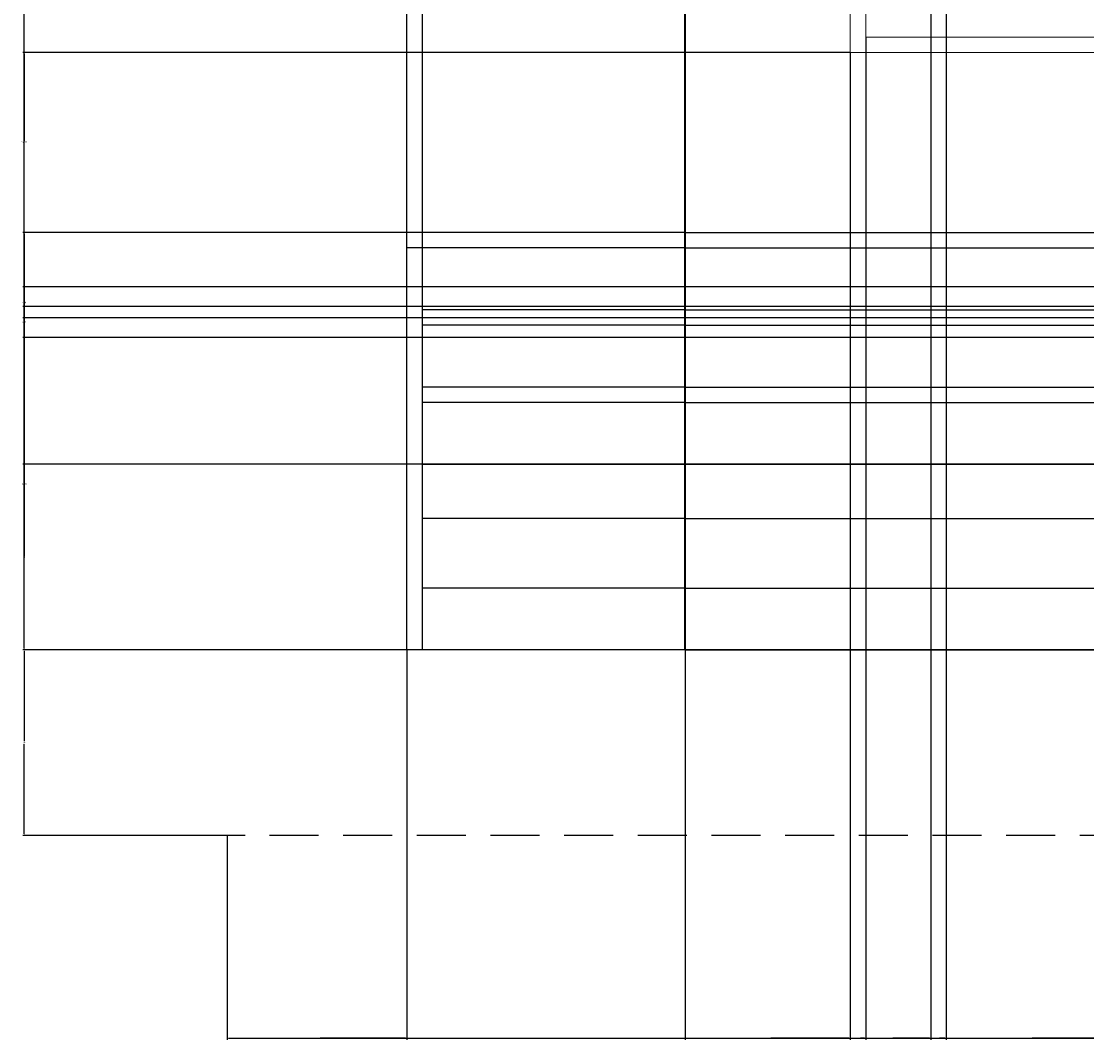
# Model space of a CAD drawing. Units: inches. Extents: x 1817 to 2378, y 1915 to 2370.
# Tile 1 of 8: x 1817 to 1955, y 1915 to 2047. Entities that reach past the tile are written whole.
import ezdxf

# ---------------------------------------------------------------- set-up
doc = ezdxf.new("R2010")
doc.units = ezdxf.units.IN
doc.linetypes.add('DASHED', pattern=[19.05, 12.7, -6.35])
doc.linetypes.add('DASHED2', pattern=[9.525, 6.35, -3.175])
for name, color, linetype, lineweight in [('A-ANNO-DIMS', 2, 'Continuous', 18), ('A-ELEV', 7, 'Continuous', 35), ('A-ELEV-HIDN', 8, 'DASHED', 18), ('A-FLOR-STRS', 3, 'Continuous', 25), ('A-GLAZ', 4, 'Continuous', 18), ('C-TOPO', 8, 'DASHED2', 25)]:
    doc.layers.add(name, color=color, linetype=linetype, lineweight=lineweight)
doc.styles.get("Standard").update_dxf_attribs({"font": 'arial.ttf'})
doc.dimstyles.get("Standard").update_dxf_attribs({"dimtxt": 0.18, "dimasz": 0.18, "dimexe": 0.18, "dimexo": 0.0625, "dimgap": 0.09, "dimtad": 0, "dimtih": 1, "dimtoh": 1, "dimdec": 4, "dimzin": 0, "dimdsep": 46, "dimtxsty": 'Standard', "dimcen": 0.09, "dimadec": 0, "dimazin": 0, "dimtfac": 1, "dimtdec": 4, "dimtofl": 0, "dimtmove": 0, "dimatfit": 3, "dimfxl": 1, "dimtolj": 1, "dimtzin": 0, "dimarcsym": 0})

# ---------------------------------------------------------------- blocks, each defined once
blk = doc.blocks.new('WIN-SQ-900')
for points in [[(1924.43, 2204.58), (1960.43, 2204.58), (1960.43, 2217.58), (1924.43, 2217.58)], [(1924.43, 2204.58), (1960.43, 2204.58), (1960.43, 2168.58), (1924.43, 2168.58)], [(1926.43, 2202.58), (1958.43, 2202.58), (1958.43, 2170.58), (1926.43, 2170.58)]]:
    blk.add_lwpolyline(points, close=True)
blk = doc.blocks.new('*D10')
at = {"layer": 'A-ANNO-DIMS', "color": 0, "lineweight": -2, "transparency": 16777216}
for p, q in [((1867.08, 2019.57), (1867.08, 2369.94)), ((1867.26, 2369.76), (1884.87, 2369.76)), ((1902.9, 2369.76), (1885.3, 2369.76)), ((1903.08, 2019.57), (1903.08, 2369.94))]:
    blk.add_line(p, q, dxfattribs=at)
at = {"layer": 'A-ANNO-DIMS', "color": 0, "transparency": 16777216}
for points in [[(1867.26, 2369.79), (1867.26, 2369.73), (1867.08, 2369.76)], [(1902.9, 2369.79), (1902.9, 2369.73), (1903.08, 2369.76)]]:
    blk.add_solid(points, dxfattribs=at)
at = {"layer": 'Defpoints', "color": 0, "transparency": 16777216}
for p in [(1903.08, 2369.76), (1867.08, 2019.51), (1903.08, 2019.51)]:
    blk.add_point(p, dxfattribs=at)
at = {"layer": 'A-ANNO-DIMS', "color": 0, "transparency": 16777216, "insert": (1885.08, 2369.76), "char_height": 0.18, "attachment_point": 5}
blk.add_mtext('\\A1;36', dxfattribs=at)
blk = doc.blocks.new('*D12')
at = {"layer": 'A-ANNO-DIMS', "color": 0, "lineweight": -2, "transparency": 16777216}
for p, q in [((1924.43, 2042.72), (1924.43, 1915.08)), ((1903.08, 2019.45), (1903.08, 1915.08)), ((1903.26, 1915.26), (1913.36, 1915.26)), ((1924.25, 1915.26), (1914.15, 1915.26))]:
    blk.add_line(p, q, dxfattribs=at)
at = {"layer": 'A-ANNO-DIMS', "color": 0, "transparency": 16777216}
for points in [[(1903.26, 1915.29), (1903.26, 1915.23), (1903.08, 1915.26)], [(1924.25, 1915.29), (1924.25, 1915.23), (1924.43, 1915.26)]]:
    blk.add_solid(points, dxfattribs=at)
at = {"layer": 'Defpoints', "color": 0, "transparency": 16777216}
for p in [(1924.43, 2042.79), (1903.08, 2019.51), (1924.43, 1915.26)]:
    blk.add_point(p, dxfattribs=at)
at = {"layer": 'A-ANNO-DIMS', "color": 0, "transparency": 16777216, "insert": (1913.76, 1915.26), "char_height": 0.18, "attachment_point": 5}
blk.add_mtext('\\A1;21.34', dxfattribs=at)
blk = doc.blocks.new('*D13')
at = {"layer": 'A-ANNO-DIMS', "color": 0, "lineweight": -2, "transparency": 16777216}
for p, q in [((1934.83, 2100.21), (1934.83, 1915.08)), ((1924.43, 2042.72), (1924.43, 1915.08)), ((1924.61, 1915.26), (1929.31, 1915.26)), ((1934.65, 1915.26), (1929.94, 1915.26))]:
    blk.add_line(p, q, dxfattribs=at)
at = {"layer": 'A-ANNO-DIMS', "color": 0, "transparency": 16777216}
for points in [[(1924.61, 1915.29), (1924.61, 1915.23), (1924.43, 1915.26)], [(1934.65, 1915.29), (1934.65, 1915.23), (1934.83, 1915.26)]]:
    blk.add_solid(points, dxfattribs=at)
at = {"layer": 'Defpoints', "color": 0, "transparency": 16777216}
for p in [(1934.83, 2100.28), (1924.43, 2042.79), (1934.83, 1915.26)]:
    blk.add_point(p, dxfattribs=at)
at = {"layer": 'A-ANNO-DIMS', "color": 0, "transparency": 16777216, "insert": (1929.63, 1915.26), "char_height": 0.18, "attachment_point": 5}
blk.add_mtext('\\A1;10.4', dxfattribs=at)
blk = doc.blocks.new('*D14')
at = {"layer": 'A-ANNO-DIMS', "color": 0, "lineweight": -2, "transparency": 16777216}
for p, q in [((1934.83, 2100.21), (1934.83, 1915.08)), ((1960.43, 2042.72), (1960.43, 1915.08)), ((1935.01, 1915.26), (1947.3, 1915.26)), ((1960.25, 1915.26), (1947.95, 1915.26))]:
    blk.add_line(p, q, dxfattribs=at)
at = {"layer": 'A-ANNO-DIMS', "color": 0, "transparency": 16777216}
for points in [[(1935.01, 1915.29), (1935.01, 1915.23), (1934.83, 1915.26)], [(1960.25, 1915.29), (1960.25, 1915.23), (1960.43, 1915.26)]]:
    blk.add_solid(points, dxfattribs=at)
at = {"layer": 'Defpoints', "color": 0, "transparency": 16777216}
for p in [(1934.83, 2100.28), (1960.43, 2042.79), (1960.43, 1915.26)]:
    blk.add_point(p, dxfattribs=at)
at = {"layer": 'A-ANNO-DIMS', "color": 0, "transparency": 16777216, "insert": (1947.63, 1915.26), "char_height": 0.18, "attachment_point": 5}
blk.add_mtext('\\A1;25.6', dxfattribs=at)
blk = doc.blocks.new('*D23')
at = {"layer": 'A-ANNO-DIMS', "color": 0, "lineweight": -2, "transparency": 16777216}
for p, q in [((2320.11, 2156.45), (2320.11, 1915.08)), ((1867.08, 1965.45), (1867.08, 1915.08)), ((1867.26, 1915.26), (2093.3, 1915.26)), ((2319.93, 1915.26), (2093.89, 1915.26))]:
    blk.add_line(p, q, dxfattribs=at)
at = {"layer": 'A-ANNO-DIMS', "color": 0, "transparency": 16777216}
for points in [[(1867.26, 1915.29), (1867.26, 1915.23), (1867.08, 1915.26)], [(2319.93, 1915.29), (2319.93, 1915.23), (2320.11, 1915.26)]]:
    blk.add_solid(points, dxfattribs=at)
at = {"layer": 'Defpoints', "color": 0, "transparency": 16777216}
for p in [(2320.11, 2156.51), (1867.08, 1965.51), (2320.11, 1915.26)]:
    blk.add_point(p, dxfattribs=at)
at = {"layer": 'A-ANNO-DIMS', "color": 0, "transparency": 16777216, "insert": (2093.6, 1915.26), "char_height": 0.18, "attachment_point": 5}
blk.add_mtext('\\A1;453', dxfattribs=at)
blk = doc.blocks.new('*D53')
at = {"layer": 'A-ANNO-DIMS', "color": 0, "lineweight": -2, "transparency": 16777216}
for p, q in [((1867.02, 1965.51), (1817.4, 1965.51)), ((1817.58, 1965.33), (1817.58, 1953.69)), ((1817.58, 1941.69), (1817.58, 1953.33)), ((1843.77, 1941.51), (1817.4, 1941.51))]:
    blk.add_line(p, q, dxfattribs=at)
at = {"layer": 'A-ANNO-DIMS', "color": 0, "transparency": 16777216}
for points in [[(1817.55, 1965.33), (1817.61, 1965.33), (1817.58, 1965.51)], [(1817.55, 1941.69), (1817.61, 1941.69), (1817.58, 1941.51)]]:
    blk.add_solid(points, dxfattribs=at)
at = {"layer": 'Defpoints', "color": 0, "transparency": 16777216}
for p in [(1817.58, 1965.51), (1867.08, 1965.51), (1843.83, 1941.51)]:
    blk.add_point(p, dxfattribs=at)
at = {"layer": 'A-ANNO-DIMS', "color": 0, "transparency": 16777216, "insert": (1817.58, 1953.51), "char_height": 0.18, "attachment_point": 5}
blk.add_mtext('\\A1;24', dxfattribs=at)
blk = doc.blocks.new('*D54')
at = {"layer": 'A-ANNO-DIMS', "color": 0, "lineweight": -2, "transparency": 16777216}
for p, q in [((1901.02, 2343.51), (1817.4, 2343.51)), ((1817.58, 2343.33), (1817.58, 2154.69)), ((1817.58, 1965.69), (1817.58, 2154.33)), ((1867.02, 1965.51), (1817.4, 1965.51))]:
    blk.add_line(p, q, dxfattribs=at)
at = {"layer": 'A-ANNO-DIMS', "color": 0, "transparency": 16777216}
for points in [[(1817.55, 2343.33), (1817.61, 2343.33), (1817.58, 2343.51)], [(1817.55, 1965.69), (1817.61, 1965.69), (1817.58, 1965.51)]]:
    blk.add_solid(points, dxfattribs=at)
at = {"layer": 'Defpoints', "color": 0, "transparency": 16777216}
for p in [(1817.58, 2343.51), (1901.08, 2343.51), (1867.08, 1965.51)]:
    blk.add_point(p, dxfattribs=at)
at = {"layer": 'A-ANNO-DIMS', "color": 0, "transparency": 16777216, "insert": (1817.58, 2154.51), "char_height": 0.18, "attachment_point": 5}
blk.add_mtext('\\A1;378', dxfattribs=at)
blk = doc.blocks.new('*D55')
at = {"layer": 'A-ANNO-DIMS', "color": 0, "lineweight": -2, "transparency": 16777216}
for p, q in [((1903.02, 1989.51), (1817.4, 1989.51)), ((1817.58, 1989.33), (1817.58, 1977.69)), ((1817.58, 1965.69), (1817.58, 1977.33)), ((1867.02, 1965.51), (1817.4, 1965.51))]:
    blk.add_line(p, q, dxfattribs=at)
at = {"layer": 'A-ANNO-DIMS', "color": 0, "transparency": 16777216}
for points in [[(1817.55, 1989.33), (1817.61, 1989.33), (1817.58, 1989.51)], [(1817.55, 1965.69), (1817.61, 1965.69), (1817.58, 1965.51)]]:
    blk.add_solid(points, dxfattribs=at)
at = {"layer": 'Defpoints', "color": 0, "transparency": 16777216}
for p in [(1817.58, 1989.51), (1903.08, 1989.51), (1867.08, 1965.51)]:
    blk.add_point(p, dxfattribs=at)
at = {"layer": 'A-ANNO-DIMS', "color": 0, "transparency": 16777216, "insert": (1817.58, 1977.51), "char_height": 0.18, "attachment_point": 5}
blk.add_mtext('\\A1;24', dxfattribs=at)
blk = doc.blocks.new('*D56')
at = {"layer": 'A-ANNO-DIMS', "color": 0, "lineweight": -2, "transparency": 16777216}
for p, q in [((1867.02, 2019.51), (1817.4, 2019.51)), ((1817.58, 2019.33), (1817.58, 2004.69)), ((1817.58, 1989.69), (1817.58, 2004.33)), ((1903.02, 1989.51), (1817.4, 1989.51))]:
    blk.add_line(p, q, dxfattribs=at)
at = {"layer": 'A-ANNO-DIMS', "color": 0, "transparency": 16777216}
for points in [[(1817.55, 2019.33), (1817.61, 2019.33), (1817.58, 2019.51)], [(1817.55, 1989.69), (1817.61, 1989.69), (1817.58, 1989.51)]]:
    blk.add_solid(points, dxfattribs=at)
at = {"layer": 'Defpoints', "color": 0, "transparency": 16777216}
for p in [(1817.58, 2019.51), (1867.08, 2019.51), (1903.08, 1989.51)]:
    blk.add_point(p, dxfattribs=at)
at = {"layer": 'A-ANNO-DIMS', "color": 0, "transparency": 16777216, "insert": (1817.58, 2004.51), "char_height": 0.18, "attachment_point": 5}
blk.add_mtext('\\A1;30', dxfattribs=at)
blk = doc.blocks.new('*D57')
at = {"layer": 'A-ANNO-DIMS', "color": 0, "lineweight": -2, "transparency": 16777216}
for p, q in [((1924.36, 2042.79), (1817.4, 2042.79)), ((1817.58, 2042.61), (1817.58, 2031.33)), ((1817.58, 2019.69), (1817.58, 2030.97)), ((1867.02, 2019.51), (1817.4, 2019.51))]:
    blk.add_line(p, q, dxfattribs=at)
at = {"layer": 'A-ANNO-DIMS', "color": 0, "transparency": 16777216}
for points in [[(1817.55, 2042.61), (1817.61, 2042.61), (1817.58, 2042.79)], [(1817.55, 2019.69), (1817.61, 2019.69), (1817.58, 2019.51)]]:
    blk.add_solid(points, dxfattribs=at)
at = {"layer": 'Defpoints', "color": 0, "transparency": 16777216}
for p in [(1817.58, 2042.79), (1924.43, 2042.79), (1867.08, 2019.51)]:
    blk.add_point(p, dxfattribs=at)
at = {"layer": 'A-ANNO-DIMS', "color": 0, "transparency": 16777216, "insert": (1817.58, 2031.15), "char_height": 0.18, "attachment_point": 5}
blk.add_mtext('\\A1;23.277', dxfattribs=at)
blk = doc.blocks.new('*D80')
at = {"layer": 'A-ANNO-DIMS', "color": 0, "lineweight": -2, "transparency": 16777216}
for p, q in [((2123.56, 2008.45), (1817.4, 2008.45)), ((1817.58, 2008.27), (1817.58, 1987.16)), ((1817.58, 1965.69), (1817.58, 1986.8)), ((2281.02, 1965.51), (1817.4, 1965.51))]:
    blk.add_line(p, q, dxfattribs=at)
at = {"layer": 'A-ANNO-DIMS', "color": 0, "transparency": 16777216}
for points in [[(1817.55, 2008.27), (1817.61, 2008.27), (1817.58, 2008.45)], [(1817.55, 1965.69), (1817.61, 1965.69), (1817.58, 1965.51)]]:
    blk.add_solid(points, dxfattribs=at)
at = {"layer": 'Defpoints', "color": 0, "transparency": 16777216}
for p in [(1817.58, 2008.45), (2123.62, 2008.45), (2281.08, 1965.51)]:
    blk.add_point(p, dxfattribs=at)
at = {"layer": 'A-ANNO-DIMS', "color": 0, "transparency": 16777216, "insert": (1817.58, 1986.98), "char_height": 0.18, "attachment_point": 5}
blk.add_mtext('\\A1;42.94', dxfattribs=at)
blk = doc.blocks.new('*D83')
at = {"layer": 'A-ANNO-DIMS', "color": 0, "lineweight": -2, "transparency": 16777216}
for p, q in [((1936.83, 2102.21), (1936.83, 1915.08)), ((1934.83, 2100.21), (1934.83, 1915.08)), ((1935.01, 1915.26), (1935.68, 1915.26)), ((1936.65, 1915.26), (1935.98, 1915.26))]:
    blk.add_line(p, q, dxfattribs=at)
at = {"layer": 'A-ANNO-DIMS', "color": 0, "transparency": 16777216}
for points in [[(1935.01, 1915.29), (1935.01, 1915.23), (1934.83, 1915.26)], [(1936.65, 1915.29), (1936.65, 1915.23), (1936.83, 1915.26)]]:
    blk.add_solid(points, dxfattribs=at)
at = {"layer": 'Defpoints', "color": 0, "transparency": 16777216}
for p in [(1936.83, 2102.28), (1934.83, 2100.28), (1936.83, 1915.26)]:
    blk.add_point(p, dxfattribs=at)
at = {"layer": 'A-ANNO-DIMS', "color": 0, "transparency": 16777216, "insert": (1935.83, 1915.26), "char_height": 0.18, "attachment_point": 5}
blk.add_mtext('\\A1;2', dxfattribs=at)
blk = doc.blocks.new('*D87')
at = {"layer": 'A-ANNO-DIMS', "color": 0, "lineweight": -2, "transparency": 16777216}
for p, q in [((1926.43, 2044.72), (1926.43, 1915.08)), ((1924.43, 2042.72), (1924.43, 1915.08)), ((1924.61, 1915.26), (1925.1, 1915.26)), ((1926.25, 1915.26), (1925.75, 1915.26))]:
    blk.add_line(p, q, dxfattribs=at)
at = {"layer": 'A-ANNO-DIMS', "color": 0, "transparency": 16777216}
for points in [[(1924.61, 1915.29), (1924.61, 1915.23), (1924.43, 1915.26)], [(1926.25, 1915.29), (1926.25, 1915.23), (1926.43, 1915.26)]]:
    blk.add_solid(points, dxfattribs=at)
at = {"layer": 'Defpoints', "color": 0, "transparency": 16777216}
for p in [(1926.43, 2044.79), (1924.43, 2042.79), (1926.43, 1915.26)]:
    blk.add_point(p, dxfattribs=at)
at = {"layer": 'A-ANNO-DIMS', "color": 0, "transparency": 16777216, "insert": (1925.43, 1915.26), "char_height": 0.18, "attachment_point": 5}
blk.add_mtext('\\A1;2.00', dxfattribs=at)
blk = doc.blocks.new('*D88')
at = {"layer": 'A-ANNO-DIMS', "color": 0, "lineweight": -2, "transparency": 16777216}
for p, q in [((1936.83, 2102.21), (1936.83, 1915.08)), ((1934.83, 2100.21), (1934.83, 1915.08)), ((1935.01, 1915.26), (1935.5, 1915.26)), ((1936.65, 1915.26), (1936.15, 1915.26))]:
    blk.add_line(p, q, dxfattribs=at)
at = {"layer": 'A-ANNO-DIMS', "color": 0, "transparency": 16777216}
for points in [[(1935.01, 1915.29), (1935.01, 1915.23), (1934.83, 1915.26)], [(1936.65, 1915.29), (1936.65, 1915.23), (1936.83, 1915.26)]]:
    blk.add_solid(points, dxfattribs=at)
at = {"layer": 'Defpoints', "color": 0, "transparency": 16777216}
for p in [(1936.83, 2102.28), (1934.83, 2100.28), (1936.83, 1915.26)]:
    blk.add_point(p, dxfattribs=at)
at = {"layer": 'A-ANNO-DIMS', "color": 0, "transparency": 16777216, "insert": (1935.83, 1915.26), "char_height": 0.18, "attachment_point": 5}
blk.add_mtext('\\A1;2.00', dxfattribs=at)
blk = doc.blocks.new('*D92')
at = {"layer": 'A-ANNO-DIMS', "color": 0, "lineweight": -2, "transparency": 16777216}
for p, q in [((2127.56, 2012.45), (1817.4, 2012.45)), ((1817.58, 2012.27), (1817.58, 2010.63)), ((1817.58, 2008.63), (1817.58, 2010.26)), ((2123.56, 2008.45), (1817.4, 2008.45))]:
    blk.add_line(p, q, dxfattribs=at)
at = {"layer": 'A-ANNO-DIMS', "color": 0, "transparency": 16777216}
for points in [[(1817.55, 2012.27), (1817.61, 2012.27), (1817.58, 2012.45)], [(1817.55, 2008.63), (1817.61, 2008.63), (1817.58, 2008.45)]]:
    blk.add_solid(points, dxfattribs=at)
at = {"layer": 'Defpoints', "color": 0, "transparency": 16777216}
for p in [(2127.62, 2012.45), (1817.58, 2008.45), (2123.62, 2008.45)]:
    blk.add_point(p, dxfattribs=at)
at = {"layer": 'A-ANNO-DIMS', "color": 0, "transparency": 16777216, "insert": (1817.58, 2010.45), "char_height": 0.18, "attachment_point": 5}
blk.add_mtext('\\A1;4.00', dxfattribs=at)
blk = doc.blocks.new('*D96')
at = {"layer": 'A-ANNO-DIMS', "color": 0, "lineweight": -2, "transparency": 16777216}
for p, q in [((2214.55, 2009.93), (1817.4, 2009.93)), ((1817.58, 2009.75), (1817.58, 2008.11)), ((1817.58, 2006.11), (1817.58, 2007.75)), ((2210.55, 2005.93), (1817.4, 2005.93))]:
    blk.add_line(p, q, dxfattribs=at)
at = {"layer": 'A-ANNO-DIMS', "color": 0, "transparency": 16777216}
for points in [[(1817.55, 2009.75), (1817.61, 2009.75), (1817.58, 2009.93)], [(1817.55, 2006.11), (1817.61, 2006.11), (1817.58, 2005.93)]]:
    blk.add_solid(points, dxfattribs=at)
at = {"layer": 'Defpoints', "color": 0, "transparency": 16777216}
for p in [(2214.62, 2009.93), (1817.58, 2005.93), (2210.62, 2005.93)]:
    blk.add_point(p, dxfattribs=at)
at = {"layer": 'A-ANNO-DIMS', "color": 0, "transparency": 16777216, "insert": (1817.58, 2007.93), "char_height": 0.18, "attachment_point": 5}
blk.add_mtext('\\A1;4.00', dxfattribs=at)
blk = doc.blocks.new('*D107')
at = {"layer": 'A-ANNO-DIMS', "color": 0, "lineweight": -2, "transparency": 16777216}
for p, q in [((1903.15, 2019.51), (2377.4, 2019.51)), ((2377.22, 2019.33), (2377.22, 2018.69)), ((1903.15, 2017.51), (2377.4, 2017.51)), ((2377.22, 2017.69), (2377.22, 2018.33))]:
    blk.add_line(p, q, dxfattribs=at)
at = {"layer": 'A-ANNO-DIMS', "color": 0, "transparency": 16777216}
for points in [[(2377.19, 2019.33), (2377.25, 2019.33), (2377.22, 2019.51)], [(2377.19, 2017.69), (2377.25, 2017.69), (2377.22, 2017.51)]]:
    blk.add_solid(points, dxfattribs=at)
at = {"layer": 'Defpoints', "color": 0, "transparency": 16777216}
for p in [(1903.08, 2019.51), (1903.08, 2017.51), (2377.22, 2017.51)]:
    blk.add_point(p, dxfattribs=at)
at = {"layer": 'A-ANNO-DIMS', "color": 0, "transparency": 16777216, "insert": (2377.22, 2018.51), "char_height": 0.18, "attachment_point": 5}
blk.add_mtext('\\A1;2.00', dxfattribs=at)
blk = doc.blocks.new('*D108')
at = {"layer": 'A-ANNO-DIMS', "color": 0, "lineweight": -2, "transparency": 16777216}
for p, q in [((1903.15, 2017.51), (2377.4, 2017.51)), ((2377.22, 2017.33), (2377.22, 2013.69)), ((2377.22, 2009.69), (2377.22, 2013.33)), ((1903.15, 2009.51), (2377.4, 2009.51))]:
    blk.add_line(p, q, dxfattribs=at)
at = {"layer": 'A-ANNO-DIMS', "color": 0, "transparency": 16777216}
for points in [[(2377.19, 2017.33), (2377.25, 2017.33), (2377.22, 2017.51)], [(2377.19, 2009.69), (2377.25, 2009.69), (2377.22, 2009.51)]]:
    blk.add_solid(points, dxfattribs=at)
at = {"layer": 'Defpoints', "color": 0, "transparency": 16777216}
for p in [(1903.08, 2017.51), (1903.08, 2009.51), (2377.22, 2009.51)]:
    blk.add_point(p, dxfattribs=at)
at = {"layer": 'A-ANNO-DIMS', "color": 0, "transparency": 16777216, "insert": (2377.22, 2013.51), "char_height": 0.18, "attachment_point": 5}
blk.add_mtext('\\A1;8.00', dxfattribs=at)
blk = doc.blocks.new('*D109')
at = {"layer": 'A-ANNO-DIMS', "color": 0, "lineweight": -2, "transparency": 16777216}
for p, q in [((1903.15, 2009.51), (2377.4, 2009.51)), ((2377.22, 2009.33), (2377.22, 2008.69)), ((2377.22, 2007.69), (2377.22, 2008.33)), ((1903.15, 2007.51), (2377.4, 2007.51))]:
    blk.add_line(p, q, dxfattribs=at)
at = {"layer": 'A-ANNO-DIMS', "color": 0, "transparency": 16777216}
for points in [[(2377.19, 2009.33), (2377.25, 2009.33), (2377.22, 2009.51)], [(2377.19, 2007.69), (2377.25, 2007.69), (2377.22, 2007.51)]]:
    blk.add_solid(points, dxfattribs=at)
at = {"layer": 'Defpoints', "color": 0, "transparency": 16777216}
for p in [(1903.08, 2009.51), (1903.08, 2007.51), (2377.22, 2007.51)]:
    blk.add_point(p, dxfattribs=at)
at = {"layer": 'A-ANNO-DIMS', "color": 0, "transparency": 16777216, "insert": (2377.22, 2008.51), "char_height": 0.18, "attachment_point": 5}
blk.add_mtext('\\A1;2.00', dxfattribs=at)
blk = doc.blocks.new('*D110')
at = {"layer": 'A-ANNO-DIMS', "color": 0, "lineweight": -2, "transparency": 16777216}
for p, q in [((1903.15, 2007.51), (2377.4, 2007.51)), ((2377.22, 2007.33), (2377.22, 2003.69)), ((2377.22, 1999.69), (2377.22, 2003.33)), ((1903.15, 1999.51), (2377.4, 1999.51))]:
    blk.add_line(p, q, dxfattribs=at)
at = {"layer": 'A-ANNO-DIMS', "color": 0, "transparency": 16777216}
for points in [[(2377.19, 2007.33), (2377.25, 2007.33), (2377.22, 2007.51)], [(2377.19, 1999.69), (2377.25, 1999.69), (2377.22, 1999.51)]]:
    blk.add_solid(points, dxfattribs=at)
at = {"layer": 'Defpoints', "color": 0, "transparency": 16777216}
for p in [(1903.08, 2007.51), (1903.08, 1999.51), (2377.22, 1999.51)]:
    blk.add_point(p, dxfattribs=at)
at = {"layer": 'A-ANNO-DIMS', "color": 0, "transparency": 16777216, "insert": (2377.22, 2003.51), "char_height": 0.18, "attachment_point": 5}
blk.add_mtext('\\A1;8.00', dxfattribs=at)
blk = doc.blocks.new('*D111')
at = {"layer": 'A-ANNO-DIMS', "color": 0, "lineweight": -2, "transparency": 16777216}
for p, q in [((1903.15, 1999.51), (2377.4, 1999.51)), ((2377.22, 1999.33), (2377.22, 1998.69)), ((2377.22, 1997.69), (2377.22, 1998.33)), ((1903.15, 1997.51), (2377.4, 1997.51))]:
    blk.add_line(p, q, dxfattribs=at)
at = {"layer": 'A-ANNO-DIMS', "color": 0, "transparency": 16777216}
for points in [[(2377.19, 1999.33), (2377.25, 1999.33), (2377.22, 1999.51)], [(2377.19, 1997.69), (2377.25, 1997.69), (2377.22, 1997.51)]]:
    blk.add_solid(points, dxfattribs=at)
at = {"layer": 'Defpoints', "color": 0, "transparency": 16777216}
for p in [(1903.08, 1999.51), (1903.08, 1997.51), (2377.22, 1997.51)]:
    blk.add_point(p, dxfattribs=at)
at = {"layer": 'A-ANNO-DIMS', "color": 0, "transparency": 16777216, "insert": (2377.22, 1998.51), "char_height": 0.18, "attachment_point": 5}
blk.add_mtext('\\A1;2.00', dxfattribs=at)
blk = doc.blocks.new('*D112')
at = {"layer": 'A-ANNO-DIMS', "color": 0, "lineweight": -2, "transparency": 16777216}
for p, q in [((1903.15, 1997.51), (2377.4, 1997.51)), ((2377.22, 1997.33), (2377.22, 1993.69)), ((2377.22, 1989.69), (2377.22, 1993.33)), ((1903.15, 1989.51), (2377.4, 1989.51))]:
    blk.add_line(p, q, dxfattribs=at)
at = {"layer": 'A-ANNO-DIMS', "color": 0, "transparency": 16777216}
for points in [[(2377.19, 1997.33), (2377.25, 1997.33), (2377.22, 1997.51)], [(2377.19, 1989.69), (2377.25, 1989.69), (2377.22, 1989.51)]]:
    blk.add_solid(points, dxfattribs=at)
at = {"layer": 'Defpoints', "color": 0, "transparency": 16777216}
for p in [(1903.08, 1997.51), (1903.08, 1989.51), (2377.22, 1989.51)]:
    blk.add_point(p, dxfattribs=at)
at = {"layer": 'A-ANNO-DIMS', "color": 0, "transparency": 16777216, "insert": (2377.22, 1993.51), "char_height": 0.18, "attachment_point": 5}
blk.add_mtext('\\A1;8.00', dxfattribs=at)
blk = doc.blocks.new('*D113')
at = {"layer": 'A-ANNO-DIMS', "color": 0, "lineweight": -2, "transparency": 16777216}
for p, q in [((1903.15, 1989.51), (2377.4, 1989.51)), ((2377.22, 1989.33), (2377.22, 1986.19)), ((2377.22, 1982.69), (2377.22, 1985.83)), ((1903.15, 1982.51), (2377.4, 1982.51))]:
    blk.add_line(p, q, dxfattribs=at)
at = {"layer": 'A-ANNO-DIMS', "color": 0, "transparency": 16777216}
for points in [[(2377.19, 1989.33), (2377.25, 1989.33), (2377.22, 1989.51)], [(2377.19, 1982.69), (2377.25, 1982.69), (2377.22, 1982.51)]]:
    blk.add_solid(points, dxfattribs=at)
at = {"layer": 'Defpoints', "color": 0, "transparency": 16777216}
for p in [(1903.08, 1989.51), (1903.08, 1982.51), (2377.22, 1982.51)]:
    blk.add_point(p, dxfattribs=at)
at = {"layer": 'A-ANNO-DIMS', "color": 0, "transparency": 16777216, "insert": (2377.22, 1986.01), "char_height": 0.18, "attachment_point": 5}
blk.add_mtext('\\A1;7.00', dxfattribs=at)
blk = doc.blocks.new('*D114')
at = {"layer": 'A-ANNO-DIMS', "color": 0, "lineweight": -2, "transparency": 16777216}
for p, q in [((1903.15, 1982.51), (2377.4, 1982.51)), ((2377.22, 1982.33), (2377.22, 1978.19)), ((2377.22, 1973.69), (2377.22, 1977.83)), ((1903.15, 1973.51), (2377.4, 1973.51))]:
    blk.add_line(p, q, dxfattribs=at)
at = {"layer": 'A-ANNO-DIMS', "color": 0, "transparency": 16777216}
for points in [[(2377.19, 1982.33), (2377.25, 1982.33), (2377.22, 1982.51)], [(2377.19, 1973.69), (2377.25, 1973.69), (2377.22, 1973.51)]]:
    blk.add_solid(points, dxfattribs=at)
at = {"layer": 'Defpoints', "color": 0, "transparency": 16777216}
for p in [(1903.08, 1982.51), (1903.08, 1973.51), (2377.22, 1973.51)]:
    blk.add_point(p, dxfattribs=at)
at = {"layer": 'A-ANNO-DIMS', "color": 0, "transparency": 16777216, "insert": (2377.22, 1978.01), "char_height": 0.18, "attachment_point": 5}
blk.add_mtext('\\A1;9.00', dxfattribs=at)
blk = doc.blocks.new('*D115')
at = {"layer": 'A-ANNO-DIMS', "color": 0, "lineweight": -2, "transparency": 16777216}
for p, q in [((1903.15, 1973.51), (2377.4, 1973.51)), ((2377.22, 1973.33), (2377.22, 1969.69)), ((2377.22, 1965.69), (2377.22, 1969.33)), ((1903.15, 1965.51), (2377.4, 1965.51))]:
    blk.add_line(p, q, dxfattribs=at)
at = {"layer": 'A-ANNO-DIMS', "color": 0, "transparency": 16777216}
for points in [[(2377.19, 1973.33), (2377.25, 1973.33), (2377.22, 1973.51)], [(2377.19, 1965.69), (2377.25, 1965.69), (2377.22, 1965.51)]]:
    blk.add_solid(points, dxfattribs=at)
at = {"layer": 'Defpoints', "color": 0, "transparency": 16777216}
for p in [(1903.08, 1973.51), (1903.08, 1965.51), (2377.22, 1965.51)]:
    blk.add_point(p, dxfattribs=at)
at = {"layer": 'A-ANNO-DIMS', "color": 0, "transparency": 16777216, "insert": (2377.22, 1969.51), "char_height": 0.18, "attachment_point": 5}
blk.add_mtext('\\A1;8.00', dxfattribs=at)
blk = doc.blocks.new('*D116')
at = {"layer": 'A-ANNO-DIMS', "color": 0, "lineweight": -2, "transparency": 16777216}
for p, q in [((1867.08, 2017.57), (1867.08, 2369.94)), ((1867.26, 2369.76), (1867.76, 2369.76)), ((1868.9, 2369.76), (1868.41, 2369.76)), ((1869.08, 2017.57), (1869.08, 2369.94))]:
    blk.add_line(p, q, dxfattribs=at)
at = {"layer": 'A-ANNO-DIMS', "color": 0, "transparency": 16777216}
for points in [[(1867.26, 2369.79), (1867.26, 2369.73), (1867.08, 2369.76)], [(1868.9, 2369.79), (1868.9, 2369.73), (1869.08, 2369.76)]]:
    blk.add_solid(points, dxfattribs=at)
at = {"layer": 'Defpoints', "color": 0, "transparency": 16777216}
for p in [(1869.08, 2369.76), (1867.08, 2017.51), (1869.08, 2017.51)]:
    blk.add_point(p, dxfattribs=at)
at = {"layer": 'A-ANNO-DIMS', "color": 0, "transparency": 16777216, "insert": (1868.08, 2369.76), "char_height": 0.18, "attachment_point": 5}
blk.add_mtext('\\A1;2.00', dxfattribs=at)
blk = doc.blocks.new('*D117')
at = {"layer": 'A-ANNO-DIMS', "color": 0, "lineweight": -2, "transparency": 16777216}
for p, q in [((1867.08, 1965.45), (1867.08, 1915.08)), ((1843.83, 1941.45), (1843.83, 1915.08)), ((1844.01, 1915.26), (1855.06, 1915.26)), ((1866.9, 1915.26), (1855.86, 1915.26))]:
    blk.add_line(p, q, dxfattribs=at)
at = {"layer": 'A-ANNO-DIMS', "color": 0, "transparency": 16777216}
for points in [[(1844.01, 1915.29), (1844.01, 1915.23), (1843.83, 1915.26)], [(1866.9, 1915.29), (1866.9, 1915.23), (1867.08, 1915.26)]]:
    blk.add_solid(points, dxfattribs=at)
at = {"layer": 'Defpoints', "color": 0, "transparency": 16777216}
for p in [(1867.08, 1965.51), (1843.83, 1941.51), (1867.08, 1915.26)]:
    blk.add_point(p, dxfattribs=at)
at = {"layer": 'A-ANNO-DIMS', "color": 0, "transparency": 16777216, "insert": (1855.46, 1915.26), "char_height": 0.18, "attachment_point": 5}
blk.add_mtext('\\A1;23.25', dxfattribs=at)
blk = doc.blocks.new('*D118')
at = {"layer": 'A-ANNO-DIMS', "color": 0, "lineweight": -2, "transparency": 16777216}
for p, q in [((1843.83, 1941.45), (1843.83, 1915.08)), ((2350.97, 1941.45), (2350.97, 1915.08)), ((1844.01, 1915.26), (2096.94, 1915.26)), ((2350.79, 1915.26), (2097.86, 1915.26))]:
    blk.add_line(p, q, dxfattribs=at)
at = {"layer": 'A-ANNO-DIMS', "color": 0, "transparency": 16777216}
for points in [[(1844.01, 1915.29), (1844.01, 1915.23), (1843.83, 1915.26)], [(2350.79, 1915.29), (2350.79, 1915.23), (2350.97, 1915.26)]]:
    blk.add_solid(points, dxfattribs=at)
at = {"layer": 'Defpoints', "color": 0, "transparency": 16777216}
for p in [(1843.83, 1941.51), (2350.97, 1941.51), (2350.97, 1915.26)]:
    blk.add_point(p, dxfattribs=at)
at = {"layer": 'A-ANNO-DIMS', "color": 0, "transparency": 16777216, "insert": (2097.4, 1915.26), "char_height": 0.18, "attachment_point": 5}
blk.add_mtext('\\A1;507.13', dxfattribs=at)
blk = doc.blocks.new('*D119')
at = {"layer": 'A-ANNO-DIMS', "color": 0, "lineweight": -2, "transparency": 16777216}
for p, q in [((1903.08, 1989.57), (1903.08, 2369.94)), ((1903.26, 2369.76), (2091.62, 2369.76)), ((2280.9, 2369.76), (2092.55, 2369.76)), ((2281.08, 1989.57), (2281.08, 2369.94))]:
    blk.add_line(p, q, dxfattribs=at)
at = {"layer": 'A-ANNO-DIMS', "color": 0, "transparency": 16777216}
for points in [[(1903.26, 2369.79), (1903.26, 2369.73), (1903.08, 2369.76)], [(2280.9, 2369.79), (2280.9, 2369.73), (2281.08, 2369.76)]]:
    blk.add_solid(points, dxfattribs=at)
at = {"layer": 'Defpoints', "color": 0, "transparency": 16777216}
for p in [(2281.08, 2369.76), (1903.08, 1989.51), (2281.08, 1989.51)]:
    blk.add_point(p, dxfattribs=at)
at = {"layer": 'A-ANNO-DIMS', "color": 0, "transparency": 16777216, "insert": (2092.08, 2369.76), "char_height": 0.18, "attachment_point": 5}
blk.add_mtext('\\A1;378.00', dxfattribs=at)
blk = doc.blocks.new('*D120')
at = {"layer": 'A-ANNO-DIMS', "color": 0, "lineweight": -2, "transparency": 16777216}
for p, q in [((1983.02, 2117.51), (1817.4, 2117.51)), ((1817.58, 2117.33), (1817.58, 2053.69)), ((1817.58, 1989.69), (1817.58, 2053.33)), ((1983.02, 1989.51), (1817.4, 1989.51))]:
    blk.add_line(p, q, dxfattribs=at)
at = {"layer": 'A-ANNO-DIMS', "color": 0, "transparency": 16777216}
for points in [[(1817.55, 2117.33), (1817.61, 2117.33), (1817.58, 2117.51)], [(1817.55, 1989.69), (1817.61, 1989.69), (1817.58, 1989.51)]]:
    blk.add_solid(points, dxfattribs=at)
at = {"layer": 'Defpoints', "color": 0, "transparency": 16777216}
for p in [(1817.58, 2117.51), (1983.08, 2117.51), (1983.08, 1989.51)]:
    blk.add_point(p, dxfattribs=at)
at = {"layer": 'A-ANNO-DIMS', "color": 0, "transparency": 16777216, "insert": (1817.58, 2053.51), "char_height": 0.18, "attachment_point": 5}
blk.add_mtext('\\A1;128.00', dxfattribs=at)

msp = doc.modelspace()

# ---------------------------------------------------------------- linework, layer by layer
at = {"layer": 'A-ELEV'}
msp.add_line((1903.0849, 1965.5087), (1903.0849, 2117.5087), dxfattribs=at)
at = {"layer": 'A-ELEV-HIDN'}
msp.add_line((2281.0849, 1989.5087), (1903.0849, 1989.5087), dxfattribs=at)
at = {"layer": 'A-FLOR-STRS'}
for p, q in [((1867.0849, 1965.5087), (1867.0849, 2019.5087)), ((1903.0849, 2019.5087), (1867.0849, 2019.5087)), ((1903.0849, 2017.5087), (1867.0849, 2017.5087)), ((1869.0849, 1965.5087), (1869.0849, 2017.5087)), ((1903.0849, 2009.5087), (1869.0849, 2009.5087)), ((1903.0849, 2007.5087), (1869.0849, 2007.5087)), ((1903.0849, 1999.5087), (1869.0849, 1999.5087)), ((1903.0849, 1997.5087), (1869.0849, 1997.5087)), ((1903.0849, 1989.5087), (1869.0849, 1989.5087)), ((1903.0849, 1982.5087), (1869.0849, 1982.5087)), ((1903.0849, 1973.5087), (1869.0849, 1973.5087))]:
    msp.add_line(p, q, dxfattribs=at)
at = {"layer": 'C-TOPO'}
for p, q in [((1867.0849, 1965.5087), (1843.834, 1965.5087)), ((2281.0849, 1965.5087), (1867.0849, 1965.5087)), ((2350.9681, 1941.5087), (1843.834, 1941.5087))]:
    msp.add_line(p, q, dxfattribs=at)

# ---------------------------------------------------------------- block references
at = {"layer": 'A-GLAZ'}
msp.add_blockref('WIN-SQ-900', (0, -125.7955), dxfattribs=at)

# ---------------------------------------------------------------- dimensions: what is measured, and where the dimension line sits
at = {"layer": 'A-ANNO-DIMS'}
for base, p1, p2, override, picture, middle in [((1903.0849, 2369.7587), (1867.0849, 2019.5087), (1903.0849, 2019.5087), {"dimdec": 0, "dimlfac": 1, "dimrnd": 0, "dimzin": 0, "dimdsep": 46, "dimlunit": 2}, '*D10', (1885.0849, 2369.7587)), ((1869.0849, 2369.7587), (1867.0849, 2017.5087), (1869.0849, 2017.5087), {"dimdec": 2, "dimlfac": 1, "dimrnd": 0, "dimzin": 0, "dimdsep": 46, "dimlunit": 2}, '*D116', (1868.0849, 2369.7587)), ((2281.0849, 2369.7587), (1903.0849, 1989.5087), (2281.0849, 1989.5087), {"dimdec": 2, "dimlfac": 1, "dimrnd": 0, "dimzin": 0, "dimdsep": 46, "dimlunit": 2}, '*D119', (2092.0849, 2369.7587)), ((2320.1054, 1915.2587), (1867.0849, 1965.5087), (2320.1054, 2156.5133), {"dimdec": 0, "dimlfac": 1, "dimrnd": 0, "dimzin": 0, "dimdsep": 46, "dimlunit": 2}, '*D23', (2093.5951, 1915.2587)), ((1936.8265, 1915.2587), (1934.8265, 2100.2756), (1936.8265, 2102.2756), {"dimdec": 0, "dimlfac": 1, "dimrnd": 0, "dimzin": 0, "dimdsep": 46, "dimlunit": 2}, '*D83', (1935.8265, 1915.2587)), ((1936.8265, 1915.2587), (1934.8265, 2100.2756), (1936.8265, 2102.2756), {"dimdec": 2, "dimlfac": 1, "dimrnd": 0, "dimzin": 0, "dimdsep": 46, "dimlunit": 2}, '*D88', (1935.8265, 1915.2587)), ((1934.8265, 1915.2587), (1924.4258, 2042.7858), (1934.8265, 2100.2756), {"dimdec": 1, "dimlfac": 1, "dimrnd": 0, "dimzin": 0, "dimdsep": 46, "dimlunit": 2}, '*D13', (1929.6262, 1915.2587)), ((1960.4258, 1915.2587), (1934.8265, 2100.2756), (1960.4258, 2042.7858), {"dimdec": 1, "dimlfac": 1, "dimrnd": 0, "dimzin": 0, "dimdsep": 46, "dimlunit": 2}, '*D14', (1947.6262, 1915.2587)), ((1926.4258, 1915.2587), (1924.4258, 2042.7858), (1926.4258, 2044.7858), {"dimdec": 2, "dimlfac": 1, "dimrnd": 0, "dimzin": 0, "dimdsep": 46, "dimlunit": 2}, '*D87', (1925.4258, 1915.2587)), ((1924.4258, 1915.2587), (1903.0849, 2019.5087), (1924.4258, 2042.7858), {"dimdec": 2, "dimlfac": 1, "dimrnd": 0, "dimzin": 0, "dimdsep": 46, "dimlunit": 2}, '*D12', (1913.7553, 1915.2587)), ((1867.0849, 1915.2587), (1843.834, 1941.5087), (1867.0849, 1965.5087), {"dimdec": 2, "dimlfac": 1, "dimrnd": 0, "dimzin": 0, "dimdsep": 46, "dimlunit": 2}, '*D117', (1855.4594, 1915.2587)), ((2350.9681, 1915.2587), (1843.834, 1941.5087), (2350.9681, 1941.5087), {"dimdec": 2, "dimlfac": 1, "dimrnd": 0, "dimzin": 0, "dimdsep": 46, "dimlunit": 2}, '*D118', (2097.401, 1915.2587))]:
    dim = msp.add_linear_dim(base=base, p1=p1, p2=p2, dimstyle='Standard', override=override, dxfattribs=at)
    dim.commit()
    dim.dimension.update_dxf_attribs({"geometry": picture, "text_midpoint": middle})
for base, p1, p2, override, picture, middle in [((1817.584, 2343.5087), (1867.0849, 1965.5087), (1901.0849, 2343.5087), {"dimdec": 0, "dimlfac": 1, "dimrnd": 0, "dimzin": 0, "dimdsep": 46, "dimlunit": 2}, '*D54', (1817.584, 2154.5087)), ((1817.584, 2117.5087), (1983.0849, 1989.5087), (1983.0849, 2117.5087), {"dimdec": 2, "dimlfac": 1, "dimrnd": 0, "dimzin": 0, "dimdsep": 46, "dimlunit": 2}, '*D120', (1817.584, 2053.5087)), ((1817.584, 2042.7858), (1867.0849, 2019.5087), (1924.4258, 2042.7858), {"dimdec": 3, "dimlfac": 1, "dimrnd": 0, "dimzin": 0, "dimdsep": 46, "dimlunit": 2}, '*D57', (1817.584, 2031.1473)), ((1817.584, 2019.5087), (1903.0849, 1989.5087), (1867.0849, 2019.5087), {"dimdec": 0, "dimlfac": 1, "dimrnd": 0, "dimzin": 0, "dimdsep": 46, "dimlunit": 2}, '*D56', (1817.584, 2004.5087)), ((2377.2181, 2017.5087), (1903.0849, 2019.5087), (1903.0849, 2017.5087), {"dimdec": 2, "dimlfac": 1, "dimrnd": 0, "dimzin": 0, "dimdsep": 46, "dimlunit": 2}, '*D107', (2377.2181, 2018.5087)), ((2377.2181, 2009.5087), (1903.0849, 2017.5087), (1903.0849, 2009.5087), {"dimdec": 2, "dimlfac": 1, "dimrnd": 0, "dimzin": 0, "dimdsep": 46, "dimlunit": 2}, '*D108', (2377.2181, 2013.5087)), ((1817.584, 2008.4468), (2127.6179, 2012.4468), (2123.6179, 2008.4468), {"dimdec": 2, "dimlfac": 1, "dimrnd": 0, "dimzin": 0, "dimdsep": 46, "dimlunit": 2}, '*D92', (1817.584, 2010.4468)), ((1817.584, 2005.9313), (2214.6163, 2009.9313), (2210.6163, 2005.9313), {"dimdec": 2, "dimlfac": 1, "dimrnd": 0, "dimzin": 0, "dimdsep": 46, "dimlunit": 2}, '*D96', (1817.584, 2007.9313)), ((2377.2181, 2007.5087), (1903.0849, 2009.5087), (1903.0849, 2007.5087), {"dimdec": 2, "dimlfac": 1, "dimrnd": 0, "dimzin": 0, "dimdsep": 46, "dimlunit": 2}, '*D109', (2377.2181, 2008.5087)), ((1817.584, 2008.4468), (2281.0849, 1965.5087), (2123.6179, 2008.4468), {"dimdec": 2, "dimlfac": 1, "dimrnd": 0, "dimzin": 0, "dimdsep": 46, "dimlunit": 2}, '*D80', (1817.584, 1986.9777)), ((2377.2181, 1999.5087), (1903.0849, 2007.5087), (1903.0849, 1999.5087), {"dimdec": 2, "dimlfac": 1, "dimrnd": 0, "dimzin": 0, "dimdsep": 46, "dimlunit": 2}, '*D110', (2377.2181, 2003.5087)), ((2377.2181, 1997.5087), (1903.0849, 1999.5087), (1903.0849, 1997.5087), {"dimdec": 2, "dimlfac": 1, "dimrnd": 0, "dimzin": 0, "dimdsep": 46, "dimlunit": 2}, '*D111', (2377.2181, 1998.5087)), ((2377.2181, 1989.5087), (1903.0849, 1997.5087), (1903.0849, 1989.5087), {"dimdec": 2, "dimlfac": 1, "dimrnd": 0, "dimzin": 0, "dimdsep": 46, "dimlunit": 2}, '*D112', (2377.2181, 1993.5087)), ((1817.584, 1989.5087), (1867.0849, 1965.5087), (1903.0849, 1989.5087), {"dimdec": 0, "dimlfac": 1, "dimrnd": 0, "dimzin": 0, "dimdsep": 46, "dimlunit": 2}, '*D55', (1817.584, 1977.5087)), ((2377.2181, 1982.5087), (1903.0849, 1989.5087), (1903.0849, 1982.5087), {"dimdec": 2, "dimlfac": 1, "dimrnd": 0, "dimzin": 0, "dimdsep": 46, "dimlunit": 2}, '*D113', (2377.2181, 1986.0087)), ((2377.2181, 1973.5087), (1903.0849, 1982.5087), (1903.0849, 1973.5087), {"dimdec": 2, "dimlfac": 1, "dimrnd": 0, "dimzin": 0, "dimdsep": 46, "dimlunit": 2}, '*D114', (2377.2181, 1978.0087)), ((2377.2181, 1965.5087), (1903.0849, 1973.5087), (1903.0849, 1965.5087), {"dimdec": 2, "dimlfac": 1, "dimrnd": 0, "dimzin": 0, "dimdsep": 46, "dimlunit": 2}, '*D115', (2377.2181, 1969.5087)), ((1817.584, 1965.5087), (1843.834, 1941.5087), (1867.0849, 1965.5087), {"dimdec": 0, "dimlfac": 1, "dimrnd": 0, "dimzin": 0, "dimdsep": 46, "dimlunit": 2}, '*D53', (1817.584, 1953.5087))]:
    dim = msp.add_linear_dim(base=base, p1=p1, p2=p2, angle=90, dimstyle='Standard', override=override, dxfattribs=at)
    dim.commit()
    dim.dimension.update_dxf_attribs({"geometry": picture, "text_midpoint": middle})

doc.saveas('drawing.dxf')
